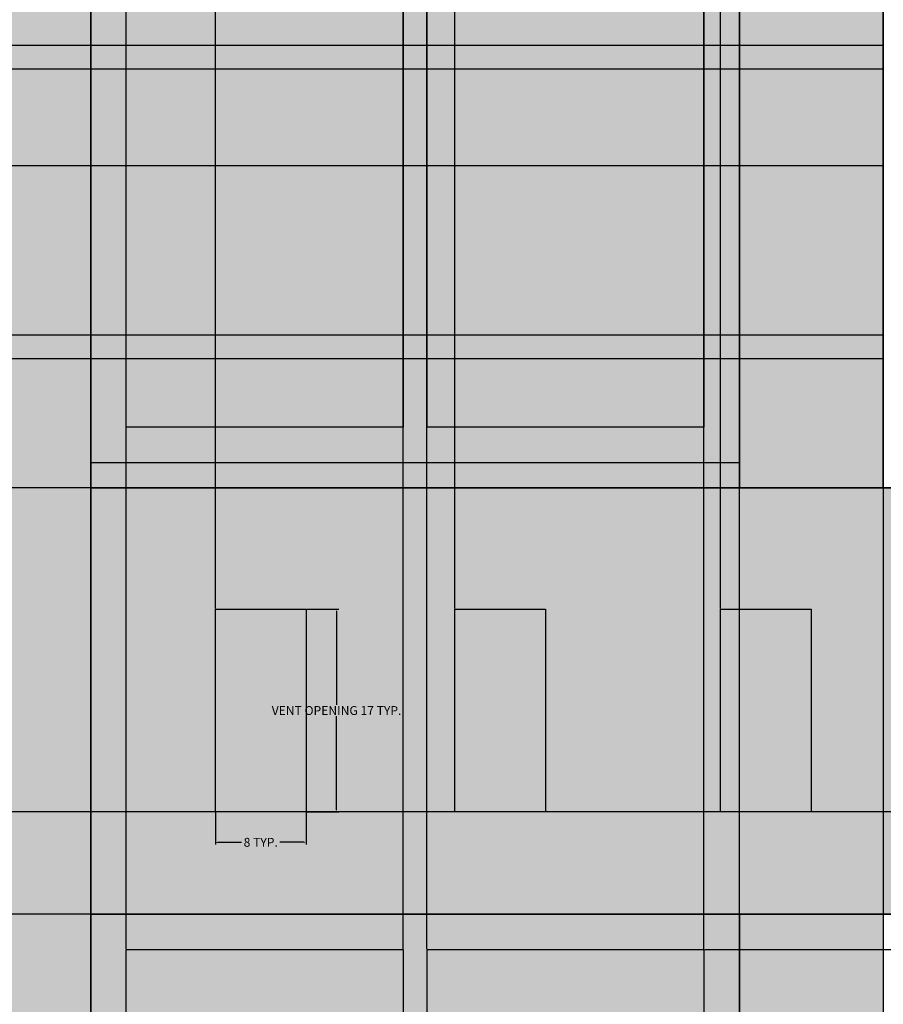
# Model space of a CAD drawing. Units: inches. Extents: x 62 to 566, y 66 to 528.
# Tile 7 of 20: x 211 to 284, y 264 to 347. Entities that reach past the tile are written whole.
import ezdxf

# ---------------------------------------------------------------- set-up
doc = ezdxf.new("R2010")
doc.units = ezdxf.units.IN
doc.header["$MEASUREMENT"] = 0
for name, color, linetype, lineweight in [('A-ANNO-DIMS', 2, 'Continuous', 18), ('A-ELEV', 7, 'Continuous', 35), ('A-GLAZ', 3, 'Continuous', 25), ('A-WALL-PATT', 8, 'Continuous', 13)]:
    doc.layers.add(name, color=color, linetype=linetype, lineweight=lineweight)
doc.styles.get("Standard").update_dxf_attribs({"font": 'arial.ttf'})
doc.dimstyles.get("Standard").update_dxf_attribs({"dimtxt": 0.75, "dimasz": 0.18, "dimexe": 0.18, "dimexo": 0.0625, "dimgap": 0.09, "dimtad": 0, "dimtih": 1, "dimtoh": 1, "dimdec": 4, "dimzin": 0, "dimdsep": 46, "dimlunit": 4, "dimtxsty": 'Standard', "dimcen": 0.09, "dimadec": 0, "dimazin": 0, "dimtfac": 1, "dimtdec": 4, "dimtofl": 0, "dimtmove": 0, "dimatfit": 3, "dimfxl": 1, "dimtolj": 1, "dimtzin": 0, "dimarcsym": 0})

# ---------------------------------------------------------------- blocks, each defined once
blk = doc.blocks.new('WIN-FRENCH-GRID')
for p, q in [((26.392, 108.058), (26.392, 83.896)), ((28.392, 108.058), (28.392, 83.896)), ((26.392, 39.969), (26.392, 3)), ((28.392, 39.969), (28.392, 3))]:
    blk.add_line(p, q)
blk.add_lwpolyline([(0, 111.058), (54.783, 111.058), (54.783, 0), (0, 0)], close=True)
for points in [[(3, 83.896), (3, 108.058), (26.392, 108.058)], [(28.392, 108.058), (51.783, 108.058), (51.783, 83.896)], [(26.392, 3), (3, 3), (3, 39.969)], [(51.783, 39.969), (51.783, 3), (28.392, 3)]]:
    blk.add_lwpolyline(points)
blk = doc.blocks.new('VENT-OPENING')
blk.add_lwpolyline([(0, 17.126), (7.664, 17.126), (7.664, 0), (0, 0)], close=True)
blk = doc.blocks.new('*D3')
at = {"layer": 'A-ANNO-DIMS', "color": 0, "lineweight": -2, "transparency": 16777216}
for p, q in [((235.527, 297.168), (238.213, 297.168)), ((238.033, 296.988), (238.033, 289.083)), ((238.033, 280.222), (238.033, 288.127)), ((235.527, 280.042), (238.213, 280.042))]:
    blk.add_line(p, q, dxfattribs=at)
at = {"layer": 'A-ANNO-DIMS', "color": 0, "transparency": 16777216}
for points in [[(238.003, 296.988), (238.063, 296.988), (238.033, 297.168)], [(238.003, 280.222), (238.063, 280.222), (238.033, 280.042)]]:
    blk.add_solid(points, dxfattribs=at)
at = {"layer": 'Defpoints', "color": 0, "transparency": 16777216}
for p in [(235.464, 297.168), (238.033, 297.168), (235.464, 280.042)]:
    blk.add_point(p, dxfattribs=at)
at = {"layer": 'A-ANNO-DIMS', "color": 0, "transparency": 16777216, "insert": (238.033, 288.605), "char_height": 0.75, "attachment_point": 5}
blk.add_mtext('\\A1;VENT OPENING 17 TYP.', dxfattribs=at)
blk = doc.blocks.new('*D4')
at = {"layer": 'A-ANNO-DIMS', "color": 0, "lineweight": -2, "transparency": 16777216}
for p, q in [((227.8, 279.98), (227.8, 277.293)), ((235.464, 279.98), (235.464, 277.293)), ((227.98, 277.473), (230.008, 277.473)), ((235.284, 277.473), (233.257, 277.473))]:
    blk.add_line(p, q, dxfattribs=at)
at = {"layer": 'A-ANNO-DIMS', "color": 0, "transparency": 16777216}
for points in [[(227.98, 277.503), (227.98, 277.443), (227.8, 277.473)], [(235.284, 277.503), (235.284, 277.443), (235.464, 277.473)]]:
    blk.add_solid(points, dxfattribs=at)
at = {"layer": 'Defpoints', "color": 0, "transparency": 16777216}
for p in [(227.8, 280.042), (235.464, 280.042), (235.464, 277.473)]:
    blk.add_point(p, dxfattribs=at)
at = {"layer": 'A-ANNO-DIMS', "color": 0, "transparency": 16777216, "insert": (231.632, 277.473), "char_height": 0.75, "attachment_point": 5}
blk.add_mtext('\\A1;8 TYP.', dxfattribs=at)
blk = doc.blocks.new('*D5')
at = {"layer": 'A-ANNO-DIMS', "color": 0, "lineweight": -2, "transparency": 16777216}
for p, q in [((272.121, 271.413), (288.897, 271.413)), ((288.717, 271.233), (288.717, 216.362)), ((288.717, 160.534), (288.717, 215.406)), ((272.121, 160.354), (288.897, 160.354))]:
    blk.add_line(p, q, dxfattribs=at)
at = {"layer": 'A-ANNO-DIMS', "color": 0, "transparency": 16777216}
for points in [[(288.687, 271.233), (288.747, 271.233), (288.717, 271.413)], [(288.687, 160.534), (288.747, 160.534), (288.717, 160.354)]]:
    blk.add_solid(points, dxfattribs=at)
at = {"layer": 'Defpoints', "color": 0, "transparency": 16777216}
for p in [(272.059, 271.413), (288.717, 271.413), (272.059, 160.354)]:
    blk.add_point(p, dxfattribs=at)
at = {"layer": 'A-ANNO-DIMS', "color": 0, "transparency": 16777216, "insert": (288.717, 215.884), "char_height": 0.75, "attachment_point": 5}
blk.add_mtext('\\A1;FRENCH WINDOW 111 TYP.', dxfattribs=at)
blk = doc.blocks.new('*D8')
at = {"layer": 'A-ANNO-DIMS', "color": 0, "lineweight": -2, "transparency": 16777216}
for p, q in [((284.202, 271.35), (284.202, 65.939)), ((125.942, 126.306), (125.942, 65.939)), ((126.122, 66.119), (203.461, 66.119)), ((284.022, 66.119), (206.683, 66.119))]:
    blk.add_line(p, q, dxfattribs=at)
at = {"layer": 'A-ANNO-DIMS', "color": 0, "transparency": 16777216}
for points in [[(126.122, 66.149), (126.122, 66.089), (125.942, 66.119)], [(284.022, 66.149), (284.022, 66.089), (284.202, 66.119)]]:
    blk.add_solid(points, dxfattribs=at)
at = {"layer": 'Defpoints', "color": 0, "transparency": 16777216}
for p in [(284.202, 271.413), (125.942, 126.369), (284.202, 66.119)]:
    blk.add_point(p, dxfattribs=at)
at = {"layer": 'A-ANNO-DIMS', "color": 0, "transparency": 16777216, "insert": (205.072, 66.119), "char_height": 0.75, "attachment_point": 5}
blk.add_mtext('\\A1;158.26', dxfattribs=at)
blk = doc.blocks.new('*D9')
at = {"layer": 'A-ANNO-DIMS', "color": 0, "lineweight": -2, "transparency": 16777216}
for p, q in [((284.202, 271.35), (284.202, 65.939)), ((316.21, 126.306), (316.21, 65.939)), ((284.382, 66.119), (298.923, 66.119)), ((316.03, 66.119), (301.489, 66.119))]:
    blk.add_line(p, q, dxfattribs=at)
at = {"layer": 'A-ANNO-DIMS', "color": 0, "transparency": 16777216}
for points in [[(284.382, 66.149), (284.382, 66.089), (284.202, 66.119)], [(316.03, 66.149), (316.03, 66.089), (316.21, 66.119)]]:
    blk.add_solid(points, dxfattribs=at)
at = {"layer": 'Defpoints', "color": 0, "transparency": 16777216}
for p in [(284.202, 271.413), (316.21, 126.369), (316.21, 66.119)]:
    blk.add_point(p, dxfattribs=at)
at = {"layer": 'A-ANNO-DIMS', "color": 0, "transparency": 16777216, "insert": (300.206, 66.119), "char_height": 0.75, "attachment_point": 5}
blk.add_mtext('\\A1;32.01', dxfattribs=at)
blk = doc.blocks.new('*D38')
at = {"layer": 'A-ANNO-DIMS', "color": 0, "lineweight": -2, "transparency": 16777216}
for p, q in [((169.043, 420.535), (169.043, 65.939)), ((217.275, 420.535), (217.275, 65.939)), ((169.223, 66.119), (191.789, 66.119)), ((217.095, 66.119), (194.53, 66.119))]:
    blk.add_line(p, q, dxfattribs=at)
at = {"layer": 'A-ANNO-DIMS', "color": 0, "transparency": 16777216}
for points in [[(169.223, 66.149), (169.223, 66.089), (169.043, 66.119)], [(217.095, 66.149), (217.095, 66.089), (217.275, 66.119)]]:
    blk.add_solid(points, dxfattribs=at)
at = {"layer": 'Defpoints', "color": 0, "transparency": 16777216}
for p in [(169.043, 420.597), (217.275, 420.597), (217.275, 66.119)]:
    blk.add_point(p, dxfattribs=at)
at = {"layer": 'A-ANNO-DIMS', "color": 0, "transparency": 16777216, "insert": (193.159, 66.119), "char_height": 0.75, "attachment_point": 5}
blk.add_mtext('\\A1;48.23', dxfattribs=at)
blk = doc.blocks.new('*D39')
at = {"layer": 'A-ANNO-DIMS', "color": 0, "lineweight": -2, "transparency": 16777216}
for p, q in [((284.202, 445.044), (284.202, 65.939)), ((217.275, 420.535), (217.275, 65.939)), ((217.455, 66.119), (249.381, 66.119)), ((284.022, 66.119), (252.096, 66.119))]:
    blk.add_line(p, q, dxfattribs=at)
at = {"layer": 'A-ANNO-DIMS', "color": 0, "transparency": 16777216}
for points in [[(217.455, 66.149), (217.455, 66.089), (217.275, 66.119)], [(284.022, 66.149), (284.022, 66.089), (284.202, 66.119)]]:
    blk.add_solid(points, dxfattribs=at)
at = {"layer": 'Defpoints', "color": 0, "transparency": 16777216}
for p in [(284.202, 445.106), (217.275, 420.597), (284.202, 66.119)]:
    blk.add_point(p, dxfattribs=at)
at = {"layer": 'A-ANNO-DIMS', "color": 0, "transparency": 16777216, "insert": (250.739, 66.119), "char_height": 0.75, "attachment_point": 5}
blk.add_mtext('\\A1;66.93', dxfattribs=at)
blk = doc.blocks.new('*D40')
at = {"layer": 'A-ANNO-DIMS', "color": 0, "lineweight": -2, "transparency": 16777216}
for p, q in [((284.202, 445.044), (284.202, 65.939)), ((316.21, 417.643), (316.21, 65.939)), ((284.382, 66.119), (298.923, 66.119)), ((316.03, 66.119), (301.489, 66.119))]:
    blk.add_line(p, q, dxfattribs=at)
at = {"layer": 'A-ANNO-DIMS', "color": 0, "transparency": 16777216}
for points in [[(284.382, 66.149), (284.382, 66.089), (284.202, 66.119)], [(316.03, 66.149), (316.03, 66.089), (316.21, 66.119)]]:
    blk.add_solid(points, dxfattribs=at)
at = {"layer": 'Defpoints', "color": 0, "transparency": 16777216}
for p in [(284.202, 445.106), (316.21, 417.706), (316.21, 66.119)]:
    blk.add_point(p, dxfattribs=at)
at = {"layer": 'A-ANNO-DIMS', "color": 0, "transparency": 16777216, "insert": (300.206, 66.119), "char_height": 0.75, "attachment_point": 5}
blk.add_mtext('\\A1;32.01', dxfattribs=at)
blk = doc.blocks.new('*D74')
at = {"layer": 'A-ANNO-DIMS', "color": 0, "lineweight": -2, "transparency": 16777216}
for p, q in [((284.202, 342.845), (284.202, 527.472)), ((284.382, 527.292), (292.858, 527.292)), ((304.636, 527.292), (296.161, 527.292)), ((304.816, 342.845), (304.816, 527.472))]:
    blk.add_line(p, q, dxfattribs=at)
at = {"layer": 'A-ANNO-DIMS', "color": 0, "transparency": 16777216}
for points in [[(284.382, 527.322), (284.382, 527.262), (284.202, 527.292)], [(304.636, 527.322), (304.636, 527.262), (304.816, 527.292)]]:
    blk.add_solid(points, dxfattribs=at)
at = {"layer": 'Defpoints', "color": 0, "transparency": 16777216}
for p in [(304.816, 527.292), (284.202, 342.782), (304.816, 342.782)]:
    blk.add_point(p, dxfattribs=at)
at = {"layer": 'A-ANNO-DIMS', "color": 0, "transparency": 16777216, "insert": (294.509, 527.292), "char_height": 0.75, "attachment_point": 5}
blk.add_mtext('\\A1;20.614', dxfattribs=at)
blk = doc.blocks.new('*D82')
at = {"layer": 'A-ANNO-DIMS', "color": 0, "lineweight": -2, "transparency": 16777216}
for p, q in [((296.375, 279.98), (296.375, 65.939)), ((284.202, 271.35), (284.202, 65.939)), ((284.382, 66.119), (288.677, 66.119)), ((296.195, 66.119), (291.9, 66.119))]:
    blk.add_line(p, q, dxfattribs=at)
at = {"layer": 'A-ANNO-DIMS', "color": 0, "transparency": 16777216}
for points in [[(284.382, 66.149), (284.382, 66.089), (284.202, 66.119)], [(296.195, 66.149), (296.195, 66.089), (296.375, 66.119)]]:
    blk.add_solid(points, dxfattribs=at)
at = {"layer": 'Defpoints', "color": 0, "transparency": 16777216}
for p in [(296.375, 280.042), (284.202, 271.413), (296.375, 66.119)]:
    blk.add_point(p, dxfattribs=at)
at = {"layer": 'A-ANNO-DIMS', "color": 0, "transparency": 16777216, "insert": (290.289, 66.119), "char_height": 0.75, "attachment_point": 5}
blk.add_mtext('\\A1;12.173', dxfattribs=at)
blk = doc.blocks.new('*D98')
at = {"layer": 'A-ANNO-DIMS', "color": 0, "lineweight": -2, "transparency": 16777216}
for p, q in [((296.313, 280.042), (63.466, 280.042)), ((63.646, 279.862), (63.646, 276.201)), ((63.646, 271.593), (63.646, 275.254)), ((284.14, 271.413), (63.466, 271.413))]:
    blk.add_line(p, q, dxfattribs=at)
at = {"layer": 'A-ANNO-DIMS', "color": 0, "transparency": 16777216}
for points in [[(63.616, 279.862), (63.676, 279.862), (63.646, 280.042)], [(63.616, 271.593), (63.676, 271.593), (63.646, 271.413)]]:
    blk.add_solid(points, dxfattribs=at)
at = {"layer": 'Defpoints', "color": 0, "transparency": 16777216}
for p in [(63.646, 280.042), (296.375, 280.042), (284.202, 271.413)]:
    blk.add_point(p, dxfattribs=at)
at = {"layer": 'A-ANNO-DIMS', "color": 0, "transparency": 16777216, "insert": (63.646, 275.728), "char_height": 0.75, "attachment_point": 5}
blk.add_mtext('\\A1;8.63', dxfattribs=at)
blk = doc.blocks.new('*D99')
at = {"layer": 'A-ANNO-DIMS', "color": 0, "lineweight": -2, "transparency": 16777216}
for p, q in [((284.14, 318.305), (63.466, 318.305)), ((63.646, 318.125), (63.646, 313.332)), ((63.646, 307.593), (63.646, 312.386)), ((284.14, 307.413), (63.466, 307.413))]:
    blk.add_line(p, q, dxfattribs=at)
at = {"layer": 'A-ANNO-DIMS', "color": 0, "transparency": 16777216}
for points in [[(63.616, 318.125), (63.676, 318.125), (63.646, 318.305)], [(63.616, 307.593), (63.676, 307.593), (63.646, 307.413)]]:
    blk.add_solid(points, dxfattribs=at)
at = {"layer": 'Defpoints', "color": 0, "transparency": 16777216}
for p in [(63.646, 318.305), (284.202, 318.305), (284.202, 307.413)]:
    blk.add_point(p, dxfattribs=at)
at = {"layer": 'A-ANNO-DIMS', "color": 0, "transparency": 16777216, "insert": (63.646, 312.859), "char_height": 0.75, "attachment_point": 5}
blk.add_mtext('\\A1;10.892', dxfattribs=at)
blk = doc.blocks.new('*D100')
at = {"layer": 'A-ANNO-DIMS', "color": 0, "lineweight": -2, "transparency": 16777216}
for p, q in [((284.14, 334.612), (63.466, 334.612)), ((63.646, 334.432), (63.646, 326.932)), ((63.646, 318.485), (63.646, 325.985)), ((284.14, 318.305), (63.466, 318.305))]:
    blk.add_line(p, q, dxfattribs=at)
at = {"layer": 'A-ANNO-DIMS', "color": 0, "transparency": 16777216}
for points in [[(63.616, 334.432), (63.676, 334.432), (63.646, 334.612)], [(63.616, 318.485), (63.676, 318.485), (63.646, 318.305)]]:
    blk.add_solid(points, dxfattribs=at)
at = {"layer": 'Defpoints', "color": 0, "transparency": 16777216}
for p in [(63.646, 334.612), (284.202, 334.612), (284.202, 318.305)]:
    blk.add_point(p, dxfattribs=at)
at = {"layer": 'A-ANNO-DIMS', "color": 0, "transparency": 16777216, "insert": (63.646, 326.458), "char_height": 0.75, "attachment_point": 5}
blk.add_mtext('\\A1;16.307', dxfattribs=at)
blk = doc.blocks.new('*D101')
at = {"layer": 'A-ANNO-DIMS', "color": 0, "lineweight": -2, "transparency": 16777216}
for p, q in [((284.14, 342.782), (63.466, 342.782)), ((63.646, 342.602), (63.646, 339.17)), ((63.646, 334.792), (63.646, 338.224)), ((284.14, 334.612), (63.466, 334.612))]:
    blk.add_line(p, q, dxfattribs=at)
at = {"layer": 'A-ANNO-DIMS', "color": 0, "transparency": 16777216}
for points in [[(63.616, 342.602), (63.676, 342.602), (63.646, 342.782)], [(63.616, 334.792), (63.676, 334.792), (63.646, 334.612)]]:
    blk.add_solid(points, dxfattribs=at)
at = {"layer": 'Defpoints', "color": 0, "transparency": 16777216}
for p in [(63.646, 342.782), (284.202, 342.782), (284.202, 334.612)]:
    blk.add_point(p, dxfattribs=at)
at = {"layer": 'A-ANNO-DIMS', "color": 0, "transparency": 16777216, "insert": (63.646, 338.697), "char_height": 0.75, "attachment_point": 5}
blk.add_mtext('\\A1;8.17', dxfattribs=at)
blk = doc.blocks.new('*D102')
at = {"layer": 'A-ANNO-DIMS', "color": 0, "lineweight": -2, "transparency": 16777216}
for p, q in [((284.14, 344.782), (63.466, 344.782)), ((63.646, 344.602), (63.646, 344.249)), ((284.14, 342.782), (63.466, 342.782)), ((63.646, 342.962), (63.646, 343.316))]:
    blk.add_line(p, q, dxfattribs=at)
at = {"layer": 'A-ANNO-DIMS', "color": 0, "transparency": 16777216}
for points in [[(63.616, 344.602), (63.676, 344.602), (63.646, 344.782)], [(63.616, 342.962), (63.676, 342.962), (63.646, 342.782)]]:
    blk.add_solid(points, dxfattribs=at)
at = {"layer": 'Defpoints', "color": 0, "transparency": 16777216}
for p in [(63.646, 344.782), (284.202, 344.782), (284.202, 342.782)]:
    blk.add_point(p, dxfattribs=at)
at = {"layer": 'A-ANNO-DIMS', "color": 0, "transparency": 16777216, "insert": (63.646, 343.782), "char_height": 0.75, "attachment_point": 5}
blk.add_mtext('\\A1;2', dxfattribs=at)
blk = doc.blocks.new('*D103')
at = {"layer": 'A-ANNO-DIMS', "color": 0, "lineweight": -2, "transparency": 16777216}
for p, q in [((284.14, 320.305), (63.466, 320.305)), ((63.646, 320.125), (63.646, 319.772)), ((63.646, 318.485), (63.646, 318.839)), ((284.14, 318.305), (63.466, 318.305))]:
    blk.add_line(p, q, dxfattribs=at)
at = {"layer": 'A-ANNO-DIMS', "color": 0, "transparency": 16777216}
for points in [[(63.616, 320.125), (63.676, 320.125), (63.646, 320.305)], [(63.616, 318.485), (63.676, 318.485), (63.646, 318.305)]]:
    blk.add_solid(points, dxfattribs=at)
at = {"layer": 'Defpoints', "color": 0, "transparency": 16777216}
for p in [(63.646, 320.305), (284.202, 320.305), (284.202, 318.305)]:
    blk.add_point(p, dxfattribs=at)
at = {"layer": 'A-ANNO-DIMS', "color": 0, "transparency": 16777216, "insert": (63.646, 319.305), "char_height": 0.75, "attachment_point": 5}
blk.add_mtext('\\A1;2', dxfattribs=at)
blk = doc.blocks.new('*D104')
at = {"layer": 'A-ANNO-DIMS', "color": 0, "lineweight": -2, "transparency": 16777216}
for p, q in [((217.275, 271.475), (217.275, 527.472)), ((217.455, 527.292), (218.44, 527.292)), ((220.095, 527.292), (219.111, 527.292)), ((220.275, 268.475), (220.275, 527.472))]:
    blk.add_line(p, q, dxfattribs=at)
at = {"layer": 'A-ANNO-DIMS', "color": 0, "transparency": 16777216}
for points in [[(217.455, 527.322), (217.455, 527.262), (217.275, 527.292)], [(220.095, 527.322), (220.095, 527.262), (220.275, 527.292)]]:
    blk.add_solid(points, dxfattribs=at)
at = {"layer": 'Defpoints', "color": 0, "transparency": 16777216}
for p in [(220.275, 527.292), (217.275, 271.413), (220.275, 268.413)]:
    blk.add_point(p, dxfattribs=at)
at = {"layer": 'A-ANNO-DIMS', "color": 0, "transparency": 16777216, "insert": (218.775, 527.292), "char_height": 0.75, "attachment_point": 5}
blk.add_mtext('\\A1;3', dxfattribs=at)
blk = doc.blocks.new('*D105')
at = {"layer": 'A-ANNO-DIMS', "color": 0, "lineweight": -2, "transparency": 16777216}
for p, q in [((220.275, 268.475), (220.275, 527.472)), ((220.455, 527.292), (230.608, 527.292)), ((243.487, 527.292), (233.334, 527.292)), ((243.667, 268.475), (243.667, 527.472))]:
    blk.add_line(p, q, dxfattribs=at)
at = {"layer": 'A-ANNO-DIMS', "color": 0, "transparency": 16777216}
for points in [[(220.455, 527.322), (220.455, 527.262), (220.275, 527.292)], [(243.487, 527.322), (243.487, 527.262), (243.667, 527.292)]]:
    blk.add_solid(points, dxfattribs=at)
at = {"layer": 'Defpoints', "color": 0, "transparency": 16777216}
for p in [(243.667, 527.292), (220.275, 268.413), (243.667, 268.413)]:
    blk.add_point(p, dxfattribs=at)
at = {"layer": 'A-ANNO-DIMS', "color": 0, "transparency": 16777216, "insert": (231.971, 527.292), "char_height": 0.75, "attachment_point": 5}
blk.add_mtext('\\A1;23.39', dxfattribs=at)
blk = doc.blocks.new('*D106')
at = {"layer": 'A-ANNO-DIMS', "color": 0, "lineweight": -2, "transparency": 16777216}
for p, q in [((243.667, 268.475), (243.667, 527.472)), ((243.847, 527.292), (244.329, 527.292)), ((245.487, 527.292), (245.005, 527.292)), ((245.667, 268.475), (245.667, 527.472))]:
    blk.add_line(p, q, dxfattribs=at)
at = {"layer": 'A-ANNO-DIMS', "color": 0, "transparency": 16777216}
for points in [[(243.847, 527.322), (243.847, 527.262), (243.667, 527.292)], [(245.487, 527.322), (245.487, 527.262), (245.667, 527.292)]]:
    blk.add_solid(points, dxfattribs=at)
at = {"layer": 'Defpoints', "color": 0, "transparency": 16777216}
for p in [(245.667, 527.292), (243.667, 268.413), (245.667, 268.413)]:
    blk.add_point(p, dxfattribs=at)
at = {"layer": 'A-ANNO-DIMS', "color": 0, "transparency": 16777216, "insert": (244.667, 527.292), "char_height": 0.75, "attachment_point": 5}
blk.add_mtext('\\A1;2', dxfattribs=at)
blk = doc.blocks.new('*D107')
at = {"layer": 'A-ANNO-DIMS', "color": 0, "lineweight": -2, "transparency": 16777216}
for p, q in [((245.667, 268.475), (245.667, 527.472)), ((245.847, 527.292), (256, 527.292)), ((268.879, 527.292), (258.725, 527.292)), ((269.059, 268.475), (269.059, 527.472))]:
    blk.add_line(p, q, dxfattribs=at)
at = {"layer": 'A-ANNO-DIMS', "color": 0, "transparency": 16777216}
for points in [[(245.847, 527.322), (245.847, 527.262), (245.667, 527.292)], [(268.879, 527.322), (268.879, 527.262), (269.059, 527.292)]]:
    blk.add_solid(points, dxfattribs=at)
at = {"layer": 'Defpoints', "color": 0, "transparency": 16777216}
for p in [(269.059, 527.292), (245.667, 268.413), (269.059, 268.413)]:
    blk.add_point(p, dxfattribs=at)
at = {"layer": 'A-ANNO-DIMS', "color": 0, "transparency": 16777216, "insert": (257.363, 527.292), "char_height": 0.75, "attachment_point": 5}
blk.add_mtext('\\A1;23.39', dxfattribs=at)
blk = doc.blocks.new('*D108')
at = {"layer": 'A-ANNO-DIMS', "color": 0, "lineweight": -2, "transparency": 16777216}
for p, q in [((269.059, 268.475), (269.059, 527.472)), ((269.239, 527.292), (270.223, 527.292)), ((271.879, 527.292), (270.894, 527.292)), ((272.059, 271.475), (272.059, 527.472))]:
    blk.add_line(p, q, dxfattribs=at)
at = {"layer": 'A-ANNO-DIMS', "color": 0, "transparency": 16777216}
for points in [[(269.239, 527.322), (269.239, 527.262), (269.059, 527.292)], [(271.879, 527.322), (271.879, 527.262), (272.059, 527.292)]]:
    blk.add_solid(points, dxfattribs=at)
at = {"layer": 'Defpoints', "color": 0, "transparency": 16777216}
for p in [(272.059, 527.292), (272.059, 271.413), (269.059, 268.413)]:
    blk.add_point(p, dxfattribs=at)
at = {"layer": 'A-ANNO-DIMS', "color": 0, "transparency": 16777216, "insert": (270.559, 527.292), "char_height": 0.75, "attachment_point": 5}
blk.add_mtext('\\A1;3', dxfattribs=at)
blk = doc.blocks.new('*D109')
at = {"layer": 'A-ANNO-DIMS', "color": 0, "lineweight": -2, "transparency": 16777216}
for p, q in [((217.275, 307.475), (217.275, 527.472)), ((217.455, 527.292), (220.923, 527.292)), ((227.62, 527.292), (224.152, 527.292)), ((227.8, 297.231), (227.8, 527.472))]:
    blk.add_line(p, q, dxfattribs=at)
at = {"layer": 'A-ANNO-DIMS', "color": 0, "transparency": 16777216}
for points in [[(217.455, 527.322), (217.455, 527.262), (217.275, 527.292)], [(227.62, 527.322), (227.62, 527.262), (227.8, 527.292)]]:
    blk.add_solid(points, dxfattribs=at)
at = {"layer": 'Defpoints', "color": 0, "transparency": 16777216}
for p in [(227.8, 527.292), (217.275, 307.413), (227.8, 297.168)]:
    blk.add_point(p, dxfattribs=at)
at = {"layer": 'A-ANNO-DIMS', "color": 0, "transparency": 16777216, "insert": (222.538, 527.292), "char_height": 0.75, "attachment_point": 5}
blk.add_mtext('\\A1;10.525', dxfattribs=at)
blk = doc.blocks.new('*D110')
at = {"layer": 'A-ANNO-DIMS', "color": 0, "lineweight": -2, "transparency": 16777216}
for p, q in [((227.8, 297.231), (227.8, 527.472)), ((227.98, 527.292), (236.256, 527.292)), ((247.834, 527.292), (239.559, 527.292)), ((248.014, 297.231), (248.014, 527.472))]:
    blk.add_line(p, q, dxfattribs=at)
at = {"layer": 'A-ANNO-DIMS', "color": 0, "transparency": 16777216}
for points in [[(227.98, 527.322), (227.98, 527.262), (227.8, 527.292)], [(247.834, 527.322), (247.834, 527.262), (248.014, 527.292)]]:
    blk.add_solid(points, dxfattribs=at)
at = {"layer": 'Defpoints', "color": 0, "transparency": 16777216}
for p in [(248.014, 527.292), (227.8, 297.168), (248.014, 297.168)]:
    blk.add_point(p, dxfattribs=at)
at = {"layer": 'A-ANNO-DIMS', "color": 0, "transparency": 16777216, "insert": (237.907, 527.292), "char_height": 0.75, "attachment_point": 5}
blk.add_mtext('\\A1;20.214', dxfattribs=at)
blk = doc.blocks.new('*D111')
at = {"layer": 'A-ANNO-DIMS', "color": 0, "lineweight": -2, "transparency": 16777216}
for p, q in [((248.014, 297.231), (248.014, 527.472)), ((248.194, 527.292), (257.867, 527.292)), ((270.263, 527.292), (260.59, 527.292)), ((270.443, 297.231), (270.443, 527.472))]:
    blk.add_line(p, q, dxfattribs=at)
at = {"layer": 'A-ANNO-DIMS', "color": 0, "transparency": 16777216}
for points in [[(248.194, 527.322), (248.194, 527.262), (248.014, 527.292)], [(270.263, 527.322), (270.263, 527.262), (270.443, 527.292)]]:
    blk.add_solid(points, dxfattribs=at)
at = {"layer": 'Defpoints', "color": 0, "transparency": 16777216}
for p in [(270.443, 527.292), (248.014, 297.168), (270.443, 297.168)]:
    blk.add_point(p, dxfattribs=at)
at = {"layer": 'A-ANNO-DIMS', "color": 0, "transparency": 16777216, "insert": (259.228, 527.292), "char_height": 0.75, "attachment_point": 5}
blk.add_mtext('\\A1;22.43', dxfattribs=at)
blk = doc.blocks.new('*D112')
at = {"layer": 'A-ANNO-DIMS', "color": 0, "lineweight": -2, "transparency": 16777216}
for p, q in [((270.443, 297.231), (270.443, 527.472)), ((270.623, 527.292), (276.002, 527.292)), ((284.022, 527.292), (278.642, 527.292)), ((284.202, 307.475), (284.202, 527.472))]:
    blk.add_line(p, q, dxfattribs=at)
at = {"layer": 'A-ANNO-DIMS', "color": 0, "transparency": 16777216}
for points in [[(270.623, 527.322), (270.623, 527.262), (270.443, 527.292)], [(284.022, 527.322), (284.022, 527.262), (284.202, 527.292)]]:
    blk.add_solid(points, dxfattribs=at)
at = {"layer": 'Defpoints', "color": 0, "transparency": 16777216}
for p in [(284.202, 527.292), (284.202, 307.413), (270.443, 297.168)]:
    blk.add_point(p, dxfattribs=at)
at = {"layer": 'A-ANNO-DIMS', "color": 0, "transparency": 16777216, "insert": (277.322, 527.292), "char_height": 0.75, "attachment_point": 5}
blk.add_mtext('\\A1;13.76', dxfattribs=at)
blk = doc.blocks.new('*D127')
at = {"layer": 'A-ANNO-DIMS', "color": 0, "lineweight": -2, "transparency": 16777216}
for p, q in [((269.121, 268.413), (564.467, 268.413)), ((564.287, 268.233), (564.287, 256.805)), ((564.287, 244.431), (564.287, 255.859)), ((269.121, 244.251), (564.467, 244.251))]:
    blk.add_line(p, q, dxfattribs=at)
at = {"layer": 'A-ANNO-DIMS', "color": 0, "transparency": 16777216}
for points in [[(564.257, 268.233), (564.317, 268.233), (564.287, 268.413)], [(564.257, 244.431), (564.317, 244.431), (564.287, 244.251)]]:
    blk.add_solid(points, dxfattribs=at)
at = {"layer": 'Defpoints', "color": 0, "transparency": 16777216}
for p in [(269.059, 268.413), (564.287, 268.413), (269.059, 244.251)]:
    blk.add_point(p, dxfattribs=at)
at = {"layer": 'A-ANNO-DIMS', "color": 0, "transparency": 16777216, "insert": (564.287, 256.332), "char_height": 0.75, "attachment_point": 5}
blk.add_mtext('\\A1;24.16', dxfattribs=at)
blk = doc.blocks.new('*D128')
at = {"layer": 'A-ANNO-DIMS', "color": 0, "lineweight": -2, "transparency": 16777216}
for p, q in [((272.121, 271.413), (564.467, 271.413)), ((564.287, 271.233), (564.287, 270.386)), ((564.287, 268.593), (564.287, 269.44)), ((269.121, 268.413), (564.467, 268.413))]:
    blk.add_line(p, q, dxfattribs=at)
at = {"layer": 'A-ANNO-DIMS', "color": 0, "transparency": 16777216}
for points in [[(564.257, 271.233), (564.317, 271.233), (564.287, 271.413)], [(564.257, 268.593), (564.317, 268.593), (564.287, 268.413)]]:
    blk.add_solid(points, dxfattribs=at)
at = {"layer": 'Defpoints', "color": 0, "transparency": 16777216}
for p in [(272.059, 271.413), (564.287, 271.413), (269.059, 268.413)]:
    blk.add_point(p, dxfattribs=at)
at = {"layer": 'A-ANNO-DIMS', "color": 0, "transparency": 16777216, "insert": (564.287, 269.913), "char_height": 0.75, "attachment_point": 5}
blk.add_mtext('\\A1;3', dxfattribs=at)
blk = doc.blocks.new('*D130')
at = {"layer": 'A-ANNO-DIMS', "color": 0, "lineweight": -2, "transparency": 16777216}
for p, q in [((227.738, 280.042), (63.466, 280.042)), ((63.646, 279.862), (63.646, 276.201)), ((63.646, 271.593), (63.646, 275.254)), ((217.213, 271.413), (63.466, 271.413))]:
    blk.add_line(p, q, dxfattribs=at)
at = {"layer": 'A-ANNO-DIMS', "color": 0, "transparency": 16777216}
for points in [[(63.616, 279.862), (63.676, 279.862), (63.646, 280.042)], [(63.616, 271.593), (63.676, 271.593), (63.646, 271.413)]]:
    blk.add_solid(points, dxfattribs=at)
at = {"layer": 'Defpoints', "color": 0, "transparency": 16777216}
for p in [(63.646, 280.042), (227.8, 280.042), (217.275, 271.413)]:
    blk.add_point(p, dxfattribs=at)
at = {"layer": 'A-ANNO-DIMS', "color": 0, "transparency": 16777216, "insert": (63.646, 275.728), "char_height": 0.75, "attachment_point": 5}
blk.add_mtext('\\A1;8.63', dxfattribs=at)

msp = doc.modelspace()

# ---------------------------------------------------------------- hatches: boundary and pattern name
at = {"layer": 'A-WALL-PATT'}
h = msp.add_hatch(color=256, dxfattribs=at)
h.dxf.hatch_style = 1
h.paths.add_polyline_path([(416.0836, 462.0423), (125.9418, 462.0423), (125.9418, 414.3686), (125.9418, 270.3686), (125.9418, 126.3686), (142.3851, 126.3686), (142.3851, 270.3686), (142.3851, 414.3686), (142.3851, 445.1064), (284.2021, 445.1064), (416.0836, 445.1064)])
h.paths.add_polyline_path([(435.3945, 503.0423), (426.3652, 503.0423), (120.4058, 503.0423), (120.4058, 501.0423), (125.9418, 501.0423), (416.0836, 501.0423), (426.3652, 501.0423), (430.6938, 501.0423), (435.3945, 501.0423)])
h.paths.add_polyline_path([(439.6878, 352.4848), (392.4793, 352.4848), (392.4793, 307.4128), (217.2752, 307.4128), (217.2752, 295.4098), (217.2752, 271.4128), (272.0586, 271.4128), (439.6878, 271.4128)])
h.paths.add_polyline_path([(248.0143, 297.1682), (255.6783, 297.1682), (255.6783, 280.0423), (248.0143, 280.0423)], flags=16)
h.paths.add_polyline_path([(235.4641, 280.0423), (227.8001, 280.0423), (227.8001, 297.1682), (235.4641, 297.1682)], flags=16)
h.paths.add_polyline_path([(270.4427, 297.1682), (278.1067, 297.1682), (278.1067, 280.0423), (270.4427, 280.0423)], flags=16)
h.paths.add_polyline_path([(296.3755, 297.1682), (304.0395, 297.1682), (304.0395, 280.0423), (296.3755, 280.0423)], flags=16)
h.paths.add_polyline_path([(319.2543, 297.1682), (326.9183, 297.1682), (326.9183, 280.0423), (319.2543, 280.0423)], flags=16)
h.paths.add_polyline_path([(341.2622, 297.1682), (348.9262, 297.1682), (348.9262, 280.0423), (341.2622, 280.0423)], flags=16)
h.paths.add_polyline_path([(389.2857, 298.3985), (433.8102, 298.3985), (433.8102, 294.9497), (389.2857, 294.9497)], flags=16)
h.paths.add_polyline_path([(389.2857, 291.6038), (433.8102, 291.6038), (433.8102, 288.155), (389.2857, 288.155)], flags=16)
h.paths.add_polyline_path([(389.2857, 284.9607), (433.8102, 284.9607), (433.8102, 281.5119), (389.2857, 281.5119)], flags=16)
h.paths.add_polyline_path([(403.5849, 311.4736), (403.5849, 317.4388), (433.1636, 317.4388), (433.1636, 311.4736)], flags=16)
h.paths.add_polyline_path([(403.5849, 323.1329), (403.5849, 329.0982), (433.1636, 329.0982), (433.1636, 323.1329)], flags=16)
h.paths.add_polyline_path([(403.5849, 334.5211), (403.5849, 340.4863), (433.1636, 340.4863), (433.1636, 334.5211)], flags=16)
h.paths.add_polyline_path([(272.0586, 160.3545), (217.2752, 160.3545), (217.2752, 129.0504), (217.2752, 126.3686), (272.0586, 126.3686)], flags=17)
h.paths.add_polyline_path([(220.5897, 149.5749), (220.5897, 152.296), (267.7931, 152.296), (267.7931, 149.5749)], flags=16)
h.paths.add_polyline_path([(267.7931, 146.6724), (267.7931, 143.9513), (220.5897, 143.9513), (220.5897, 146.6724)], flags=16)
h.paths.add_polyline_path([(220.5897, 155.3799), (220.5897, 158.101), (267.7931, 158.101), (267.7931, 155.3799)], flags=16)
h.paths.add_polyline_path([(267.7931, 140.686), (267.7931, 137.9649), (220.5897, 137.9649), (220.5897, 140.686)], flags=16)
h.paths.add_polyline_path([(267.7931, 135.516), (267.7931, 132.7949), (220.5897, 132.7949), (220.5897, 135.516)], flags=16)
h = msp.add_hatch(dxfattribs=at)
h.set_pattern_fill('ANSI36', color=256, scale=8.8)
h.paths.add_polyline_path([(217.2752, 420.597), (169.0431, 420.597), (169.0431, 126.3686), (217.2752, 126.3686), (217.2752, 129.0504), (217.2752, 271.4128), (217.2752, 295.4128), (217.2752, 307.4128)])
h.paths.add_polyline_path([(282.3509, 501.0423), (125.9418, 501.0423), (125.9418, 465.0423), (282.3509, 465.0423)])
h.paths.add_polyline_path([(209.709, 476.6506), (202.045, 476.6506), (202.045, 493.7764), (209.709, 493.7764)], flags=16)
h.paths.add_polyline_path([(193.9913, 476.6506), (186.3273, 476.6506), (186.3273, 493.7764), (193.9913, 493.7764)], flags=16)
h.paths.add_polyline_path([(177.9243, 476.6506), (170.2603, 476.6506), (170.2603, 493.7764), (177.9243, 493.7764)], flags=16)
h.paths.add_polyline_path([(163.2545, 476.3015), (155.5905, 476.3015), (155.5905, 493.4274), (163.2545, 493.4274)], flags=16)
h.paths.add_polyline_path([(148.2354, 476.3015), (140.5713, 476.3015), (140.5713, 493.4274), (148.2354, 493.4274)], flags=16)
h.paths.add_polyline_path([(284.2021, 126.3686), (87.8962, 126.3686), (87.8962, 114.3686), (87.8962, 90.3686), (284.2021, 90.3686)])
h.paths.add_polyline_path([(474.1214, 126.3686), (396.433, 126.3686), (396.433, 90.3686), (474.1214, 90.3686)])
h = msp.add_hatch(color=256, dxfattribs=at)
h.dxf.hatch_style = 1
h.paths.add_polyline_path([(416.0836, 501.0423), (282.3509, 501.0423), (282.3509, 465.0423), (416.0836, 465.0423)])
h.paths.add_polyline_path([(284.2021, 420.597), (272.0586, 420.597), (272.0586, 309.5388), (272.0586, 307.4128), (284.2021, 307.4128)], flags=17)
h.paths.add_polyline_path([(284.2021, 445.1064), (142.3851, 445.1064), (142.3851, 414.3686), (142.3851, 270.3686), (142.3851, 126.3686), (163.6548, 126.3686), (163.6548, 270.5016), (163.6548, 414.5016), (163.6548, 427.4752), (284.2021, 427.4752)])
h.paths.add_polyline_path([(235.4641, 297.1682), (227.8001, 297.1682), (227.8001, 280.0423), (235.4641, 280.0423)], flags=17)
h.paths.add_polyline_path([(255.6783, 297.1682), (248.0143, 297.1682), (248.0143, 280.0423), (255.6783, 280.0423)], flags=17)
h.paths.add_polyline_path([(278.1067, 297.1682), (270.4427, 297.1682), (270.4427, 280.0423), (278.1067, 280.0423)], flags=17)
h.paths.add_polyline_path([(304.0395, 297.1682), (296.3755, 297.1682), (296.3755, 280.0423), (304.0395, 280.0423)])
h.paths.add_polyline_path([(326.9183, 297.1682), (319.2543, 297.1682), (319.2543, 280.0423), (326.9183, 280.0423)])
h.paths.add_polyline_path([(348.9262, 297.1682), (341.2622, 297.1682), (341.2622, 280.0423), (348.9262, 280.0423)])
h.paths.add_polyline_path([(433.8102, 284.9607), (389.2857, 284.9607), (389.2857, 281.5119), (433.8102, 281.5119)])
h.paths.add_polyline_path([(433.8102, 291.6038), (389.2857, 291.6038), (389.2857, 288.155), (433.8102, 288.155)])
h.paths.add_polyline_path([(433.8102, 298.3985), (389.2857, 298.3985), (389.2857, 294.9497), (433.8102, 294.9497)])
h.paths.add_polyline_path([(433.1636, 317.4388), (403.5849, 317.4388), (403.5849, 311.4736), (433.1636, 311.4736)])
h.paths.add_polyline_path([(433.1636, 329.0982), (403.5849, 329.0982), (403.5849, 323.1329), (433.1636, 323.1329)])
h.paths.add_polyline_path([(433.1636, 340.4863), (403.5849, 340.4863), (403.5849, 334.5211), (433.1636, 334.5211)])
h.paths.add_polyline_path([(284.2021, 271.4128), (272.0586, 271.4128), (272.0586, 160.3545), (272.0586, 126.3686), (284.2021, 126.3686)])
h.paths.add_polyline_path([(267.7931, 158.101), (220.5897, 158.101), (220.5897, 155.3799), (267.7931, 155.3799)], flags=17)
h.paths.add_polyline_path([(267.7931, 152.296), (220.5897, 152.296), (220.5897, 149.5749), (267.7931, 149.5749)], flags=17)
h.paths.add_polyline_path([(267.7931, 146.6724), (220.5897, 146.6724), (220.5897, 143.9513), (267.7931, 143.9513)], flags=17)
h.paths.add_polyline_path([(267.7931, 140.686), (220.5897, 140.686), (220.5897, 137.9649), (267.7931, 137.9649)], flags=17)
h.paths.add_polyline_path([(267.7931, 135.516), (220.5897, 135.516), (220.5897, 132.7949), (267.7931, 132.7949)], flags=17)
h.paths.add_polyline_path([(148.2354, 493.4274), (140.5713, 493.4274), (140.5713, 476.3015), (148.2354, 476.3015)])
h.paths.add_polyline_path([(163.2545, 493.4274), (155.5905, 493.4274), (155.5905, 476.3015), (163.2545, 476.3015)])
h.paths.add_polyline_path([(177.9243, 493.7764), (170.2603, 493.7764), (170.2603, 476.6506), (177.9243, 476.6506)])
h.paths.add_polyline_path([(193.9913, 493.7764), (186.3273, 493.7764), (186.3273, 476.6506), (193.9913, 476.6506)])
h.paths.add_polyline_path([(209.709, 493.7764), (202.045, 493.7764), (202.045, 476.6506), (209.709, 476.6506)])
h = msp.add_hatch(color=256, dxfattribs=at)
h.dxf.hatch_style = 1
h.paths.add_polyline_path([(272.0586, 420.597), (217.2752, 420.597), (217.2752, 309.5388), (272.0586, 309.5388)])
h.paths.add_polyline_path([(245.6669, 393.435), (245.6669, 417.597), (269.0586, 417.597), (269.0586, 393.435)], flags=16)
h.paths.add_polyline_path([(245.6669, 391.435), (269.0586, 391.435), (269.0586, 351.5079), (245.6669, 351.5079)], flags=16)
h.paths.add_polyline_path([(243.6669, 393.435), (220.2752, 393.435), (220.2752, 417.597), (243.6669, 417.597)], flags=16)
h.paths.add_polyline_path([(243.6669, 391.435), (243.6669, 351.5079), (220.2752, 351.5079), (220.2752, 391.435)], flags=16)
h.paths.add_polyline_path([(245.6669, 349.5079), (269.0586, 349.5079), (269.0586, 312.5388), (245.6669, 312.5388)], flags=16)
h.paths.add_polyline_path([(243.6669, 349.5079), (243.6669, 312.5388), (220.2752, 312.5388), (220.2752, 349.5079)], flags=16)
h.paths.add_polyline_path([(272.0586, 271.4128), (217.2752, 271.4128), (217.2752, 160.3545), (272.0586, 160.3545)])
h.paths.add_polyline_path([(243.6669, 268.4128), (243.6669, 244.2507), (220.2752, 244.2507), (220.2752, 268.4128)], flags=16)
h.paths.add_polyline_path([(245.6669, 268.4128), (269.0586, 268.4128), (269.0586, 244.2507), (245.6669, 244.2507)], flags=16)
h.paths.add_polyline_path([(243.6669, 242.2507), (243.6669, 202.3236), (220.2752, 202.3236), (220.2752, 242.2507)], flags=16)
h.paths.add_polyline_path([(245.6669, 242.2507), (269.0586, 242.2507), (269.0586, 202.3236), (245.6669, 202.3236)], flags=16)
h.paths.add_polyline_path([(243.6669, 200.3236), (243.6669, 163.3545), (220.2752, 163.3545), (220.2752, 200.3236)], flags=16)
h.paths.add_polyline_path([(245.6669, 200.3236), (269.0586, 200.3236), (269.0586, 163.3545), (245.6669, 163.3545)], flags=16)
h.paths.add_polyline_path([(272.0586, 309.5388), (217.2752, 309.5388), (217.2752, 307.4128), (272.0586, 307.4128)])
h = msp.add_hatch(color=256, dxfattribs=at)
h.dxf.hatch_style = 1
h.set_gradient(color1=(0, 0, 255), color2=(0, 0, 0))
h.paths.add_polyline_path([(243.6669, 417.597), (220.2752, 417.597), (220.2752, 393.435), (243.6669, 393.435)])
h.paths.add_polyline_path([(269.0586, 417.597), (245.6669, 417.597), (245.6669, 393.435), (269.0586, 393.435)])
h.paths.add_polyline_path([(269.0586, 391.435), (245.6669, 391.435), (245.6669, 351.5079), (269.0586, 351.5079)])
h.paths.add_polyline_path([(243.6669, 391.435), (220.2752, 391.435), (220.2752, 351.5079), (243.6669, 351.5079)])
h.paths.add_polyline_path([(243.6669, 349.5079), (220.2752, 349.5079), (220.2752, 312.5388), (243.6669, 312.5388)])
h.paths.add_polyline_path([(269.0586, 349.5079), (245.6669, 349.5079), (245.6669, 312.5388), (269.0586, 312.5388)])
h.paths.add_polyline_path([(243.6669, 268.4128), (220.2752, 268.4128), (220.2752, 244.2507), (243.6669, 244.2507)])
h.paths.add_polyline_path([(269.0586, 268.4128), (245.6669, 268.4128), (245.6669, 244.2507), (269.0586, 244.2507)])
h.paths.add_polyline_path([(269.0586, 242.2507), (245.6669, 242.2507), (245.6669, 202.3236), (269.0586, 202.3236)])
h.paths.add_polyline_path([(243.6669, 242.2507), (220.2752, 242.2507), (220.2752, 202.3236), (243.6669, 202.3236)])
h.paths.add_polyline_path([(243.6669, 200.3236), (220.2752, 200.3236), (220.2752, 163.3545), (243.6669, 163.3545)])
h.paths.add_polyline_path([(269.0586, 200.3236), (245.6669, 200.3236), (245.6669, 163.3545), (269.0586, 163.3545)])
h = msp.add_hatch(color=256, dxfattribs=at)
h.dxf.hatch_style = 1
h.paths.add_polyline_path([(245.6669, 417.597), (243.6669, 417.597), (243.6669, 393.435), (220.2752, 393.435), (220.2752, 391.435), (243.6669, 391.435), (243.6669, 351.5079), (220.2752, 351.5079), (220.2752, 349.5079), (243.6669, 349.5079), (243.6669, 312.5388), (245.6669, 312.5388), (245.6669, 349.5079), (269.0586, 349.5079), (269.0586, 351.5079), (245.6669, 351.5079), (245.6669, 391.435), (269.0586, 391.435), (269.0586, 393.435), (245.6669, 393.435)], flags=0)

# ---------------------------------------------------------------- linework, layer by layer
at = {"layer": 'A-ELEV'}
for p, q in [((217.2752, 307.4128), (217.2752, 420.597)), ((272.0586, 309.5388), (272.0586, 420.597)), ((272.0586, 309.5388), (272.0586, 307.4128)), ((217.2752, 307.4128), (392.4793, 307.4128)), ((217.2752, 307.4128), (217.2752, 295.4098)), ((217.2752, 271.4128), (217.2752, 295.4128)), ((217.2752, 129.0504), (217.2752, 271.4128)), ((217.2752, 271.4128), (540.0368, 271.4128)), ((272.0586, 126.3686), (272.0586, 271.4128))]:
    msp.add_line(p, q, dxfattribs=at)

# ---------------------------------------------------------------- block references
at = {"layer": 'A-GLAZ'}
for name, p in [('WIN-FRENCH-GRID', (217.2752, 309.5388)), ('VENT-OPENING', (227.8001, 280.0423)), ('VENT-OPENING', (248.0143, 280.0423)), ('VENT-OPENING', (270.4427, 280.0423)), ('WIN-FRENCH-GRID', (217.2752, 160.3545))]:
    msp.add_blockref(name, p, dxfattribs=at)

# ---------------------------------------------------------------- dimensions: what is measured, and where the dimension line sits
at = {"layer": 'A-ANNO-DIMS'}
for base, p1, p2, override, picture, middle in [((220.2752, 527.2923), (217.2752, 271.4128), (220.2752, 268.4128), {"dimdec": 0, "dimlfac": 1, "dimrnd": 0, "dimzin": 0, "dimdsep": 46, "dimlunit": 2}, '*D104', (218.7752, 527.2923)), ((227.8001, 527.2923), (217.2752, 307.4128), (227.8001, 297.1682), {"dimdec": 3, "dimlfac": 1, "dimrnd": 0, "dimzin": 0, "dimdsep": 46, "dimlunit": 2}, '*D109', (222.5377, 527.2923)), ((243.6669, 527.2923), (220.2752, 268.4128), (243.6669, 268.4128), {"dimdec": 2, "dimlfac": 1, "dimrnd": 0, "dimzin": 0, "dimdsep": 46, "dimlunit": 2}, '*D105', (231.971, 527.2923)), ((248.0143, 527.2923), (227.8001, 297.1682), (248.0143, 297.1682), {"dimdec": 3, "dimlfac": 1, "dimrnd": 0, "dimzin": 0, "dimdsep": 46, "dimlunit": 2}, '*D110', (237.9072, 527.2923)), ((245.6669, 527.2923), (243.6669, 268.4128), (245.6669, 268.4128), {"dimdec": 0, "dimlfac": 1, "dimrnd": 0, "dimzin": 0, "dimdsep": 46, "dimlunit": 2}, '*D106', (244.6669, 527.2923)), ((269.0586, 527.2923), (245.6669, 268.4128), (269.0586, 268.4128), {"dimdec": 2, "dimlfac": 1, "dimrnd": 0, "dimzin": 0, "dimdsep": 46, "dimlunit": 2}, '*D107', (257.3627, 527.2923)), ((270.4427, 527.2923), (248.0143, 297.1682), (270.4427, 297.1682), {"dimdec": 2, "dimlfac": 1, "dimrnd": 0, "dimzin": 0, "dimdsep": 46, "dimlunit": 2}, '*D111', (259.2285, 527.2923)), ((272.0586, 527.2923), (269.0586, 268.4128), (272.0586, 271.4128), {"dimdec": 0, "dimlfac": 1, "dimrnd": 0, "dimzin": 0, "dimdsep": 46, "dimlunit": 2}, '*D108', (270.5586, 527.2923)), ((284.2021, 527.2923), (270.4427, 297.1682), (284.2021, 307.4128), {"dimdec": 2, "dimlfac": 1, "dimrnd": 0, "dimzin": 0, "dimdsep": 46, "dimlunit": 2}, '*D112', (277.3224, 527.2923)), ((304.8163, 527.2923), (284.2021, 342.7821), (304.8163, 342.7821), {"dimdec": 3, "dimlfac": 1, "dimrnd": 0, "dimzin": 0, "dimdsep": 46, "dimlunit": 2}, '*D74', (294.5092, 527.2923)), ((284.2021, 66.1186), (217.2752, 420.597), (284.2021, 445.1064), {"dimdec": 2, "dimlfac": 1, "dimrnd": 0, "dimzin": 0, "dimdsep": 46, "dimlunit": 2}, '*D39', (250.7386, 66.1186)), ((316.2101, 66.1186), (284.2021, 445.1064), (316.2101, 417.7059), {"dimdec": 2, "dimlfac": 1, "dimrnd": 0, "dimzin": 0, "dimdsep": 46, "dimlunit": 2}, '*D40', (300.2061, 66.1186)), ((217.2752, 66.1186), (169.0431, 420.597), (217.2752, 420.597), {"dimdec": 2, "dimlfac": 1, "dimrnd": 0, "dimzin": 0, "dimdsep": 46, "dimlunit": 2}, '*D38', (193.1592, 66.1186)), ((296.3755, 66.1186), (284.2021, 271.4128), (296.3755, 280.0423), {"dimdec": 3, "dimlfac": 1, "dimrnd": 0, "dimzin": 0, "dimdsep": 46, "dimlunit": 2}, '*D82', (290.2888, 66.1186)), ((284.2021, 66.1186), (125.9418, 126.3686), (284.2021, 271.4128), {"dimdec": 2, "dimlfac": 1, "dimrnd": 0, "dimzin": 0, "dimdsep": 46, "dimlunit": 2}, '*D8', (205.0719, 66.1186)), ((316.2101, 66.1186), (284.2021, 271.4128), (316.2101, 126.3686), {"dimdec": 2, "dimlfac": 1, "dimrnd": 0, "dimzin": 0, "dimdsep": 46, "dimlunit": 2}, '*D9', (300.2061, 66.1186))]:
    dim = msp.add_linear_dim(base=base, p1=p1, p2=p2, dimstyle='Standard', override=override, dxfattribs=at)
    dim.commit()
    dim.dimension.update_dxf_attribs({"geometry": picture, "text_midpoint": middle})
for base, p1, p2, override, picture, middle in [((63.6462, 344.7821), (284.2021, 342.7821), (284.2021, 344.7821), {"dimdec": 0, "dimlfac": 1, "dimrnd": 0, "dimzin": 0, "dimdsep": 46, "dimlunit": 2}, '*D102', (63.6462, 343.7821)), ((63.6462, 342.7821), (284.2021, 334.6119), (284.2021, 342.7821), {"dimdec": 2, "dimlfac": 1, "dimrnd": 0, "dimzin": 0, "dimdsep": 46, "dimlunit": 2}, '*D101', (63.6462, 338.697)), ((63.6462, 334.6119), (284.2021, 318.3051), (284.2021, 334.6119), {"dimdec": 3, "dimlfac": 1, "dimrnd": 0, "dimzin": 0, "dimdsep": 46, "dimlunit": 2}, '*D100', (63.6462, 326.4585)), ((63.6462, 320.3051), (284.2021, 318.3051), (284.2021, 320.3051), {"dimdec": 0, "dimlfac": 1, "dimrnd": 0, "dimzin": 0, "dimdsep": 46, "dimlunit": 2}, '*D103', (63.6462, 319.3051)), ((63.6462, 318.3051), (284.2021, 307.4128), (284.2021, 318.3051), {"dimdec": 3, "dimlfac": 1, "dimrnd": 0, "dimzin": 0, "dimdsep": 46, "dimlunit": 2}, '*D99', (63.6462, 312.8589)), ((63.6462, 280.0423), (284.2021, 271.4128), (296.3755, 280.0423), {"dimdec": 2, "dimlfac": 1, "dimrnd": 0, "dimzin": 0, "dimdsep": 46, "dimlunit": 2}, '*D98', (63.6462, 275.7276)), ((63.6462, 280.0423), (217.2752, 271.4128), (227.8001, 280.0423), {"dimdec": 2, "dimlfac": 1, "dimrnd": 0, "dimzin": 0, "dimdsep": 46, "dimlunit": 2}, '*D130', (63.6462, 275.7276)), ((564.2868, 271.4128), (269.0586, 268.4128), (272.0586, 271.4128), {"dimdec": 0, "dimlfac": 1, "dimrnd": 0, "dimzin": 0, "dimdsep": 46, "dimlunit": 2}, '*D128', (564.2868, 269.9128)), ((564.2868, 268.4128), (269.0586, 244.2507), (269.0586, 268.4128), {"dimdec": 2, "dimlfac": 1, "dimrnd": 0, "dimzin": 0, "dimdsep": 46, "dimlunit": 2}, '*D127', (564.2868, 256.3317))]:
    dim = msp.add_linear_dim(base=base, p1=p1, p2=p2, angle=90, dimstyle='Standard', override=override, dxfattribs=at)
    dim.commit()
    dim.dimension.update_dxf_attribs({"geometry": picture, "text_midpoint": middle})
for base, p1, p2, text, picture, middle in [((238.033, 297.1682), (235.4641, 280.0423), (235.4641, 297.1682), 'VENT OPENING <> TYP.', '*D3', (238.033, 288.6053)), ((288.7173, 271.4128), (272.0586, 160.3545), (272.0586, 271.4128), 'FRENCH WINDOW <> TYP.', '*D5', (288.7173, 215.8836))]:
    dim = msp.add_linear_dim(base=base, p1=p1, p2=p2, angle=90, text=text, dimstyle='Standard', override={"dimdec": 0, "dimlfac": 1, "dimrnd": 0, "dimzin": 0, "dimdsep": 46, "dimlunit": 2}, dxfattribs=at)
    dim.commit()
    dim.dimension.update_dxf_attribs({"geometry": picture, "text_midpoint": middle})
dim = msp.add_linear_dim(base=(235.4641, 277.4735), p1=(227.8001, 280.0423), p2=(235.4641, 280.0423), text='<> TYP.', dimstyle='Standard', override={"dimdec": 0, "dimlfac": 1, "dimrnd": 0, "dimzin": 0, "dimdsep": 46, "dimlunit": 2}, dxfattribs=at)
dim.commit()
dim.dimension.update_dxf_attribs({"geometry": '*D4', "text_midpoint": (231.6321, 277.4735)})

doc.saveas('drawing.dxf')
